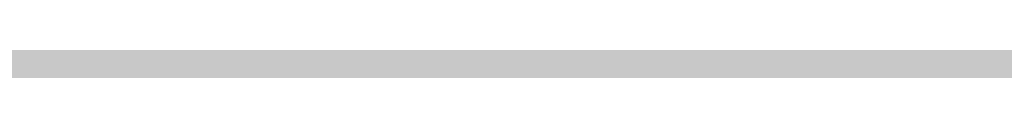
# Model space of a CAD drawing. Units: millimetres. Extents: x 0 to 2267, y 0 to 1823.
# Tile 125 of 256: x 1600.369 to 1605.705, y 1232.264 to 1232.332. Entities that reach past the tile are written whole.
import ezdxf

# ---------------------------------------------------------------- set-up
doc = ezdxf.new("R2010")
doc.units = ezdxf.units.MM
doc.header["$MEASUREMENT"] = 0
doc.layers.add('M-HATC', color=252, linetype='Continuous', lineweight=18)

msp = doc.modelspace()

# ---------------------------------------------------------------- hatches: boundary and pattern name
at = {"layer": 'M-HATC'}
h = msp.add_hatch(color=256, dxfattribs=at)
h.dxf.hatch_style = 1
h.paths.add_polyline_path([(2065.771, 1618.062, 0.236068), (2055.771, 1638.062), (1381.0868, 1638.062, 0.236068), (1371.0868, 1618.062), (1371.0868, 1603.062), (2055.771, 1603.062), (2065.771, 1603.062)])
h.paths.add_polyline_path([(2062.7718, 1550.2964), (2062.7718, 1560.2964), (1374.086, 1560.2964), (1374.086, 1550.2964), (1374.086, 1540.2964), (1384.086, 1540.2964), (1389.086, 1540.2964), (2062.7718, 1540.2964)])
h.paths.add_polyline_path([(1930.9289, 1282.7656), (1505.9289, 1282.7656), (1587.6276, 1235.5968, 0.131652), (1600.1276, 1232.2475), (1836.7302, 1232.2475, 0.131652), (1849.2302, 1235.5968)])
h.paths.add_polyline_path([(1930.9289, 1117.4171), (1905.9289, 1117.4171), (1505.9289, 1117.4171), (1505.9289, 1077.4171), (1930.9289, 1077.4171)])
h = msp.add_hatch(color=256, dxfattribs=at)
h.dxf.hatch_style = 1
h.paths.add_polyline_path([(2055.771, 1603.062), (1381.0868, 1603.062), (1381.0868, 1598.062), (2055.771, 1598.062)])
h.paths.add_polyline_path([(2055.771, 1598.062), (1381.0868, 1598.062), (1381.0868, 1593.062), (2055.771, 1593.062)])
h.paths.add_polyline_path([(2051.3074, 1536.7609), (1385.5504, 1536.7609), (1385.5504, 1526.7609), (1387.5504, 1526.7609), (1388.5366, 1525.0528), (1385.3319, 1521.2335), (1385.3319, 1521.2226), (2050.2542, 1522.7491), (2048.3212, 1525.0528), (2049.3074, 1526.7609), (2051.3074, 1526.7609)])
edge = h.paths.add_edge_path()
edge.add_arc((1847.5345, 1379.1492), 135, 222.603061, 222.890851, ccw=False)
edge.add_line((1748.1663, 1287.7656), (1683.0921, 1287.7656))
edge.add_arc((1583.7239, 1379.1492), 135, 317.109149, 317.396939, ccw=False)
edge.add_arc((1678.9686, 1290.6707), 5, 222.8909, 317.1091, ccw=False)
edge.add_arc((1774.2133, 1379.1492), 135, 222.603061, 222.890851, ccw=False)
edge.add_line((1674.8451, 1287.7656), (1609.7709, 1287.7656))
edge.add_arc((1510.4027, 1379.1492), 135, 317.109149, 317.396939, ccw=False)
edge.add_arc((1605.6474, 1290.6707), 5, 222.8909, 317.1091, ccw=False)
edge.add_arc((1700.8921, 1379.1492), 135, 222.603061, 222.890851, ccw=False)
edge.add_line((1601.5239, 1287.7656), (1536.4497, 1287.7656))
edge.add_arc((1437.0815, 1379.1492), 135, 317.109149, 317.396939, ccw=False)
edge.add_arc((1532.3262, 1290.6707), 5, 222.8909, 317.1091, ccw=False)
edge.add_arc((1627.5709, 1379.1492), 135, 222.603061, 222.890851, ccw=False)
edge.add_line((1528.2027, 1287.7656), (1505.9289, 1287.7656))
edge.add_spline(control_points=[(1505.9289, 1287.7656), (1504.2622, 1287.7656), (1504.2622, 1282.7656), (1505.9289, 1282.7656)], knot_values=[0, 0, 0, 0, 5, 5, 5, 5], degree=3, periodic=0)
edge.add_line((1505.9289, 1282.7656), (1930.9289, 1282.7656))
edge.add_spline(control_points=[(1930.9289, 1282.7656), (1932.5956, 1282.7656), (1932.5956, 1287.7656), (1930.9289, 1287.7656)], knot_values=[0, 0, 0, 0, 5, 5, 5, 5], degree=3, periodic=0)
edge.add_line((1930.9289, 1287.7656), (1903.0557, 1287.7656))
edge.add_arc((1803.6875, 1379.1492), 135, 317.109149, 317.396939, ccw=False)
edge.add_arc((1898.9322, 1290.6707), 5, 222.8909, 317.1091, ccw=False)
edge.add_arc((1994.1769, 1379.1492), 135, 222.603061, 222.890851, ccw=False)
edge.add_line((1894.8087, 1287.7656), (1829.7345, 1287.7656))
edge.add_arc((1730.3663, 1379.1492), 135, 317.109149, 317.396939, ccw=False)
edge.add_arc((1825.611, 1290.6707), 5, 222.8909, 317.1091, ccw=False)
edge.add_arc((1920.8557, 1379.1492), 135, 222.603061, 222.890851, ccw=False)
edge.add_line((1821.4875, 1287.7656), (1756.4133, 1287.7656))
edge.add_arc((1657.0451, 1379.1492), 135, 317.109149, 317.396939, ccw=False)
edge.add_arc((1752.2898, 1290.6707), 5, 222.8909, 317.1091, ccw=False)
edge = h.paths.add_edge_path()
edge.add_spline(control_points=[(1843.4289, 1227.2475), (1845.0956, 1227.2475), (1845.0956, 1232.2475), (1843.4289, 1232.2475)], knot_values=[0, 0, 0, 0, 5, 5, 5, 5], degree=3, periodic=0)
edge.add_line((1843.4289, 1232.2475), (1593.4289, 1232.2475))
edge.add_spline(control_points=[(1593.4289, 1232.2475), (1591.7622, 1232.2475), (1591.7622, 1227.2475), (1593.4289, 1227.2475)], knot_values=[0, 0, 0, 0, 5, 5, 5, 5], degree=3, periodic=0)
edge.add_line((1593.4289, 1227.2475), (1843.4289, 1227.2475))
h.paths.add_polyline_path([(1905.9289, 1127.4171), (1530.9289, 1127.4171, 0.414214), (1520.9289, 1117.4171), (1530.9289, 1117.4171), (1915.9289, 1117.4171, 0.414214)])
edge = h.paths.add_edge_path()
edge.add_arc((1397.0858, 1498.4078), 12.7299, 90.78215, 190.87871, ccw=False)
edge.add_line((1396.912, 1511.1365), (1428.0097, 1511.3488))
edge.add_line((1428.0097, 1511.3488), (1433.0097, 1511.3488))
edge.add_line((1433.0097, 1511.3488), (1434.439, 1511.3488))
edge.add_arc((1419.474, 1498.0804), 20, 41.561, 74.08211)
edge.add_line((1424.9592, 1517.3135), (1399.9351, 1517.2561))
edge.add_spline(control_points=[(1399.9307, 1517.2561), (1399.884, 1517.2131), (1399.8328, 1517.1689), (1399.7774, 1517.1236)], knot_values=[11.567499, 11.567499, 11.567499, 11.567499, 11.814249, 11.814249, 11.814249, 11.814249], degree=3, periodic=0)
edge.add_spline(control_points=[(1399.6328, 1517.0099), (1399.5831, 1516.9721), (1399.5307, 1516.9338), (1399.4759, 1516.8947)], knot_values=[11.167718, 11.167718, 11.167718, 11.167718, 11.365188, 11.365188, 11.365188, 11.365188], degree=3, periodic=0)
edge.add_spline(control_points=[(1399.3398, 1516.8001), (1399.1514, 1516.6719), (1398.9384, 1516.5377), (1398.704, 1516.3994)], knot_values=[10.376405, 10.376405, 10.376405, 10.376405, 11.00994, 11.00994, 11.00994, 11.00994], degree=3, periodic=0)
edge.add_spline(control_points=[(1398.6572, 1516.3719), (1398.5789, 1516.326), (1398.4983, 1516.2797), (1398.4155, 1516.2331)], knot_values=[10.125175, 10.125175, 10.125175, 10.125175, 10.334406, 10.334406, 10.334406, 10.334406], degree=3, periodic=0)
edge.add_spline(control_points=[(1398.2642, 1516.1487), (1398.196, 1516.1111), (1398.1263, 1516.0732), (1398.0555, 1516.0351)], knot_values=[9.832246, 9.832246, 9.832246, 9.832246, 9.999658, 9.999658, 9.999658, 9.999658], degree=3, periodic=0)
edge.add_spline(control_points=[(1397.9987, 1516.0048), (1397.7312, 1515.8621), (1397.446, 1515.7171), (1397.1466, 1515.5714)], knot_values=[9.161808, 9.161808, 9.161808, 9.161808, 9.787769, 9.787769, 9.787769, 9.787769], degree=3, periodic=0)
edge.add_spline(control_points=[(1397.1466, 1515.5714), (1396.8418, 1515.423), (1396.5222, 1515.274), (1396.1914, 1515.1262)], knot_values=[8.524455, 8.524455, 8.524455, 8.524455, 9.161808, 9.161808, 9.161808, 9.161808], degree=3, periodic=0)
edge.add_spline(control_points=[(1396.0777, 1515.0756), (1395.9854, 1515.0348), (1395.8922, 1514.994), (1395.7983, 1514.9534)], knot_values=[8.275193, 8.275193, 8.275193, 8.275193, 8.451726, 8.451726, 8.451726, 8.451726], degree=3, periodic=0)
edge.add_spline(control_points=[(1395.6018, 1514.8691), (1395.4997, 1514.8257), (1395.3968, 1514.7824), (1395.2932, 1514.7394)], knot_values=[7.962917, 7.962917, 7.962917, 7.962917, 8.152764, 8.152764, 8.152764, 8.152764], degree=3, periodic=0)
edge.add_spline(control_points=[(1395.2116, 1514.7057), (1394.8278, 1514.5475), (1394.4345, 1514.3929), (1394.0364, 1514.2442)], knot_values=[7.21254, 7.21254, 7.21254, 7.21254, 7.913148, 7.913148, 7.913148, 7.913148], degree=3, periodic=0)
edge.add_spline(control_points=[(1394.0364, 1514.2442), (1393.7076, 1514.1214), (1393.3754, 1514.0027), (1393.0427, 1513.8895)], knot_values=[6.633733, 6.633733, 6.633733, 6.633733, 7.21254, 7.21254, 7.21254, 7.21254], degree=3, periodic=0)
edge.add_spline(control_points=[(1392.8214, 1513.815), (1392.7198, 1513.7812), (1392.6181, 1513.7479), (1392.5166, 1513.7152)], knot_values=[6.328796, 6.328796, 6.328796, 6.328796, 6.505493, 6.505493, 6.505493, 6.505493], degree=3, periodic=0)
edge.add_spline(control_points=[(1392.5166, 1513.7152), (1392.3187, 1513.6515), (1392.1212, 1513.59), (1391.9244, 1513.531)], knot_values=[5.984605, 5.984605, 5.984605, 5.984605, 6.328796, 6.328796, 6.328796, 6.328796], degree=3, periodic=0)
edge.add_spline(control_points=[(1391.7915, 1513.4915), (1391.3122, 1513.3501), (1390.8384, 1513.2239), (1390.3784, 1513.1171)], knot_values=[5.066697, 5.066697, 5.066697, 5.066697, 5.907055, 5.907055, 5.907055, 5.907055], degree=3, periodic=0)
edge.add_spline(control_points=[(1390.3784, 1513.1171), (1390.1797, 1513.071), (1389.9836, 1513.0284), (1389.7907, 1512.9899)], knot_values=[4.70367, 4.70367, 4.70367, 4.70367, 5.066695, 5.066695, 5.066695, 5.066695], degree=3, periodic=0)
edge.add_spline(control_points=[(1389.422, 1512.9204), (1389.2459, 1512.8892), (1389.0729, 1512.8617), (1388.9036, 1512.8381)], knot_values=[4.130571, 4.130571, 4.130571, 4.130571, 4.469816, 4.469816, 4.469816, 4.469816], degree=3, periodic=0)
edge.add_spline(control_points=[(1388.9036, 1512.8381), (1388.591, 1512.7946), (1388.2911, 1512.7644), (1388.0071, 1512.7494)], knot_values=[3.504031, 3.504031, 3.504031, 3.504031, 4.130571, 4.130571, 4.130571, 4.130571], degree=3, periodic=0)
edge.add_spline(control_points=[(1387.9356, 1512.7459), (1387.8538, 1512.7423), (1387.7733, 1512.74), (1387.6944, 1512.739)], knot_values=[3.268866, 3.268866, 3.268866, 3.268866, 3.451164, 3.451164, 3.451164, 3.451164], degree=3, periodic=0)
edge.add_spline(control_points=[(1387.3351, 1512.7443), (1387.2076, 1512.7499), (1387.0847, 1512.7597), (1386.967, 1512.7739)], knot_values=[2.670686, 2.670686, 2.670686, 2.670686, 2.984, 2.984, 2.984, 2.984], degree=3, periodic=0)
edge.add_spline(control_points=[(1386.8327, 1512.7922), (1386.8209, 1512.7941), (1386.8092, 1512.7959), (1386.7975, 1512.7979)], knot_values=[2.516981, 2.516981, 2.516981, 2.516981, 2.549528, 2.549528, 2.549528, 2.549528], degree=3, periodic=0)
edge.add_spline(control_points=[(1386.4526, 1512.8735), (1386.4257, 1512.881), (1386.3993, 1512.889), (1386.3733, 1512.8972)], knot_values=[2.095869, 2.095869, 2.095869, 2.095869, 2.17941, 2.17941, 2.17941, 2.17941], degree=3, periodic=0)
edge.add_spline(control_points=[(1386.0691, 1513.0189), (1386.0634, 1513.0217), (1386.0577, 1513.0246), (1386.052, 1513.0275)], knot_values=[1.72453, 1.72453, 1.72453, 1.72453, 1.745933, 1.745933, 1.745933, 1.745933], degree=3, periodic=0)
edge.add_arc((1399.474, 1498.0804), 20, 131.82432, 180)
edge.add_arc((1630.3336, 1505.5484), 250.9708, 181.705176, 236.427975)
edge.add_arc((1605.3399, 1483.3044), 218.7822, 238.660829, 243.34961)
edge.add_arc((1647.0911, 1510.3592), 262.8986, 183.129836, 237.853442, ccw=False)
h.paths.add_polyline_path([(1406.5369, 1391.9644, 0.149382), (1491.5506, 1296.4418, -0.129517)], flags=17)
edge = h.paths.add_edge_path()
edge.add_arc((2037.3838, 1498.0804), 20, 0, 48.26587)
edge.add_spline(control_points=[(2050.6973, 1513.0052), (2050.6512, 1512.9847), (2050.6034, 1512.9655), (2050.5539, 1512.9477)], knot_values=[1.835652, 1.835652, 1.835652, 1.835652, 2.000781, 2.000781, 2.000781, 2.000781], degree=3, periodic=0)
edge.add_spline(control_points=[(2050.4616, 1512.9166), (2050.479, 1512.9221), (2050.4963, 1512.9277), (2050.5133, 1512.9335)], knot_values=[2.045477, 2.045477, 2.045477, 2.045477, 2.101389, 2.101389, 2.101389, 2.101389], degree=3, periodic=0)
edge.add_spline(control_points=[(2050.129, 1512.8342), (2050.1984, 1512.8473), (2050.2657, 1512.8623), (2050.3308, 1512.8792)], knot_values=[2.237629, 2.237629, 2.237629, 2.237629, 2.435841, 2.435841, 2.435841, 2.435841], degree=3, periodic=0)
edge.add_spline(control_points=[(2050.0946, 1512.8278), (2050.1061, 1512.8299), (2050.1176, 1512.832), (2050.129, 1512.8342)], knot_values=[2.435841, 2.435841, 2.435841, 2.435841, 2.468321, 2.468321, 2.468321, 2.468321], degree=3, periodic=0)
edge.add_spline(control_points=[(2049.7843, 1512.7851), (2049.8552, 1512.7922), (2049.9243, 1512.8008), (2049.9917, 1512.8109)], knot_values=[2.563852, 2.563852, 2.563852, 2.563852, 2.748541, 2.748541, 2.748541, 2.748541], degree=3, periodic=0)
edge.add_spline(control_points=[(2049.4052, 1512.7617), (2049.5364, 1512.7653), (2049.6629, 1512.773), (2049.7843, 1512.7851)], knot_values=[2.748541, 2.748541, 2.748541, 2.748541, 3.064882, 3.064882, 3.064882, 3.064882], degree=3, periodic=0)
edge.add_spline(control_points=[(2049.1698, 1512.7597), (2049.2336, 1512.7591), (2049.2965, 1512.7594), (2049.3584, 1512.7606)], knot_values=[3.102309, 3.102309, 3.102309, 3.102309, 3.2503, 3.2503, 3.2503, 3.2503], degree=3, periodic=0)
edge.add_spline(control_points=[(2048.8573, 1512.7691), (2048.9638, 1512.7638), (2049.068, 1512.7606), (2049.1698, 1512.7597)], knot_values=[3.2503, 3.2503, 3.2503, 3.2503, 3.486069, 3.486069, 3.486069, 3.486069], degree=3, periodic=0)
edge.add_spline(control_points=[(2048.6924, 1512.7789), (2048.3729, 1512.8009), (2048.0345, 1512.8411), (2047.6817, 1512.897)], knot_values=[3.606429, 3.606429, 3.606429, 3.606429, 4.2989, 4.2989, 4.2989, 4.2989], degree=3, periodic=0)
edge.add_spline(control_points=[(2047.6817, 1512.897), (2047.5458, 1512.9185), (2047.4077, 1512.9424), (2047.2678, 1512.9685)], knot_values=[4.2989, 4.2989, 4.2989, 4.2989, 4.565769, 4.565769, 4.565769, 4.565769], degree=3, periodic=0)
edge.add_spline(control_points=[(2047.2678, 1512.9685), (2047.1449, 1512.9914), (2047.0207, 1513.016), (2046.8951, 1513.0422)], knot_values=[4.565769, 4.565769, 4.565769, 4.565769, 4.799971, 4.799971, 4.799971, 4.799971], degree=3, periodic=0)
edge.add_spline(control_points=[(2046.8951, 1513.0422), (2046.5286, 1513.1188), (2046.1513, 1513.209), (2045.7676, 1513.3107)], knot_values=[4.799971, 4.799971, 4.799971, 4.799971, 5.483718, 5.483718, 5.483718, 5.483718], degree=3, periodic=0)
edge.add_spline(control_points=[(2045.7676, 1513.3107), (2045.3724, 1513.4154), (2044.9704, 1513.5322), (2044.5662, 1513.6588)], knot_values=[5.483718, 5.483718, 5.483718, 5.483718, 6.187866, 6.187866, 6.187866, 6.187866], degree=3, periodic=0)
edge.add_spline(control_points=[(2044.5662, 1513.6588), (2044.4149, 1513.7061), (2044.2633, 1513.7549), (2044.1116, 1513.8048)], knot_values=[6.187866, 6.187866, 6.187866, 6.187866, 6.451551, 6.451551, 6.451551, 6.451551], degree=3, periodic=0)
edge.add_spline(control_points=[(2044.1116, 1513.8048), (2043.9967, 1513.8427), (2043.8817, 1513.8813), (2043.7668, 1513.9205)], knot_values=[6.451551, 6.451551, 6.451551, 6.451551, 6.651434, 6.651434, 6.651434, 6.651434], degree=3, periodic=0)
edge.add_spline(control_points=[(2043.7668, 1513.9205), (2043.3716, 1514.0554), (2042.9774, 1514.1979), (2042.5886, 1514.3458)], knot_values=[6.651434, 6.651434, 6.651434, 6.651434, 7.338879, 7.338879, 7.338879, 7.338879], degree=3, periodic=0)
edge.add_spline(control_points=[(2042.5886, 1514.3458), (2042.1643, 1514.5071), (2041.7465, 1514.6749), (2041.3409, 1514.846)], knot_values=[7.338879, 7.338879, 7.338879, 7.338879, 8.089209, 8.089209, 8.089209, 8.089209], degree=3, periodic=0)
edge.add_spline(control_points=[(2041.3409, 1514.846), (2041.1028, 1514.9465), (2040.869, 1515.0481), (2040.6405, 1515.1502)], knot_values=[8.089209, 8.089209, 8.089209, 8.089209, 8.529587, 8.529587, 8.529587, 8.529587], degree=3, periodic=0)
edge.add_spline(control_points=[(2040.51, 1515.2089), (2040.0824, 1515.4022), (2039.6747, 1515.5971), (2039.295, 1515.7894)], knot_values=[8.613818, 8.613818, 8.613818, 8.613818, 9.44571, 9.44571, 9.44571, 9.44571], degree=3, periodic=0)
edge.add_spline(control_points=[(2039.295, 1515.7894), (2039.0618, 1515.9075), (2038.8391, 1516.0246), (2038.6288, 1516.1398)], knot_values=[9.44571, 9.44571, 9.44571, 9.44571, 9.956404, 9.956404, 9.956404, 9.956404], degree=3, periodic=0)
edge.add_spline(control_points=[(2038.6288, 1516.1398), (2038.5187, 1516.2001), (2038.4121, 1516.2598), (2038.309, 1516.3189)], knot_values=[9.956404, 9.956404, 9.956404, 9.956404, 10.223542, 10.223542, 10.223542, 10.223542], degree=3, periodic=0)
edge.add_spline(control_points=[(2038.309, 1516.3189), (2038.2138, 1516.3735), (2038.1216, 1516.4276), (2038.0328, 1516.481)], knot_values=[10.223542, 10.223542, 10.223542, 10.223542, 10.47051, 10.47051, 10.47051, 10.47051], degree=3, periodic=0)
edge.add_spline(control_points=[(2038.0328, 1516.481), (2037.7855, 1516.6296), (2037.5639, 1516.773), (2037.3722, 1516.909)], knot_values=[10.47051, 10.47051, 10.47051, 10.47051, 11.15767, 11.15767, 11.15767, 11.15767], degree=3, periodic=0)
edge.add_spline(control_points=[(2037.3722, 1516.909), (2037.2789, 1516.9752), (2037.1927, 1517.0396), (2037.1142, 1517.102)], knot_values=[11.15767, 11.15767, 11.15767, 11.15767, 11.49227, 11.49227, 11.49227, 11.49227], degree=3, periodic=0)
edge.add_spline(control_points=[(2036.8564, 1517.3259), (2036.9148, 1517.2692), (2036.9814, 1517.2103), (2037.0557, 1517.1492)], knot_values=[11.577341, 11.577341, 11.577341, 11.577341, 11.91035, 11.91035, 11.91035, 11.91035], degree=3, periodic=0)
edge.add_spline(control_points=[(2036.8074, 1517.3748), (2036.823, 1517.3587), (2036.8393, 1517.3424), (2036.8564, 1517.3259)], knot_values=[11.91035, 11.91035, 11.91035, 11.91035, 12.007402, 12.007402, 12.007402, 12.007402], degree=3, periodic=0)
edge.add_spline(control_points=[(2036.7017, 1517.494), (2036.7104, 1517.483), (2036.7196, 1517.4719), (2036.7291, 1517.4606)], knot_values=[12.184155, 12.184155, 12.184155, 12.184155, 12.255409, 12.255409, 12.255409, 12.255409], degree=3, periodic=0)
edge.add_spline(control_points=[(2036.6159, 1517.6205), (2036.62, 1517.613), (2036.6243, 1517.6055), (2036.6289, 1517.5979)], knot_values=[12.487913, 12.487913, 12.487913, 12.487913, 12.541035, 12.541035, 12.541035, 12.541035], degree=3, periodic=0)
edge.add_spline(control_points=[(2036.5635, 1517.786), (2036.5637, 1517.7794), (2036.5642, 1517.7726), (2036.565, 1517.7658)], knot_values=[12.911761, 12.911761, 12.911761, 12.911761, 12.968286, 12.968286, 12.968286, 12.968286], degree=3, periodic=0)
edge.add_spline(control_points=[(2036.6166, 1517.9304), (2036.6125, 1517.9259), (2036.6086, 1517.9212), (2036.6049, 1517.9165)], knot_values=[13.382527, 13.382527, 13.382527, 13.382527, 13.433791, 13.433791, 13.433791, 13.433791], degree=3, periodic=0)
edge.add_spline(control_points=[(2036.749, 1518.017), (2036.7361, 1518.0116), (2036.7239, 1518.006), (2036.7124, 1518.0002)], knot_values=[13.726299, 13.726299, 13.726299, 13.726299, 13.809928, 13.809928, 13.809928, 13.809928], degree=3, periodic=0)
edge.add_spline(control_points=[(2036.8604, 1518.0528), (2036.8386, 1518.0474), (2036.8181, 1518.0416), (2036.7988, 1518.0353)], knot_values=[13.910887, 13.910887, 13.910887, 13.910887, 14.02153, 14.02153, 14.02153, 14.02153], degree=3, periodic=0)
edge.add_line((2036.9639, 1518.0804), (2032.3838, 1518.0804))
edge.add_line((2032.3838, 1518.0804), (2027.3838, 1518.0804))
edge.add_line((2027.3838, 1518.0804), (2022.3838, 1518.0804))
edge.add_line((2022.3838, 1518.0804), (2017.3838, 1518.0804))
edge.add_arc((2017.3838, 1498.0804), 20, 90, 138.439)
edge.add_line((2002.4188, 1511.3488), (2003.8481, 1511.3488))
edge.add_line((2003.8481, 1511.3488), (2008.8481, 1511.3488))
edge.add_line((2008.8481, 1511.3488), (2039.772, 1511.1377))
edge.add_arc((2039.772, 1498.4078), 12.7299, -10.87871, 90, ccw=False)
edge.add_arc((1789.7668, 1510.3592), 262.8986, 302.146558, 356.870164, ccw=False)
edge.add_arc((1831.5179, 1483.3044), 218.7822, 296.65039, 301.339171)
edge.add_arc((1806.5242, 1505.5484), 250.9708, 303.572025, 358.294824)
h.paths.add_polyline_path([(2030.321, 1391.9644, -0.129517), (1945.3072, 1296.4418, 0.149382)], flags=17)
edge = h.paths.add_edge_path()
edge.add_spline(control_points=[(2037.2464, 1518.0821), (2037.2898, 1518.081), (2037.3355, 1518.0804), (2037.3838, 1518.0804)], knot_values=[0.000012, 0.000012, 0.000012, 0.000012, 0.144754, 0.144754, 0.144754, 0.144754], degree=3, periodic=0)
edge.add_line((2037.3357, 1518.0804), (2037.0096, 1518.0804))
edge.add_spline(control_points=[(2037.0096, 1518.0804), (2036.9822, 1518.0768), (2036.956, 1518.0727), (2036.9312, 1518.0681)], knot_values=[14.13465, 14.13465, 14.13465, 14.13465, 14.247197, 14.247197, 14.247197, 14.247197], degree=3, periodic=0)
edge.add_spline(control_points=[(2036.9312, 1518.0681), (2036.9276, 1518.0674), (2036.9241, 1518.0667), (2036.9205, 1518.0661)], knot_values=[14.118315, 14.118315, 14.118315, 14.118315, 14.13465, 14.13465, 14.13465, 14.13465], degree=3, periodic=0)
edge.add_spline(control_points=[(2036.9205, 1518.0661), (2036.9118, 1518.0644), (2036.9032, 1518.0626), (2036.8948, 1518.0608)], knot_values=[14.078086, 14.078086, 14.078086, 14.078086, 14.118315, 14.118315, 14.118315, 14.118315], degree=3, periodic=0)
edge.add_spline(control_points=[(2036.8948, 1518.0608), (2036.883, 1518.0583), (2036.8716, 1518.0556), (2036.8604, 1518.0528)], knot_values=[14.02153, 14.02153, 14.02153, 14.02153, 14.078086, 14.078086, 14.078086, 14.078086], degree=3, periodic=0)
edge.add_spline(control_points=[(2036.8604, 1518.0528), (2036.8386, 1518.0474), (2036.8181, 1518.0416), (2036.7988, 1518.0353)], knot_values=[13.910887, 13.910887, 13.910887, 13.910887, 14.02153, 14.02153, 14.02153, 14.02153], degree=3, periodic=0)
edge.add_spline(control_points=[(2036.7988, 1518.0353), (2036.7981, 1518.035), (2036.7974, 1518.0348), (2036.7967, 1518.0346)], knot_values=[13.906906, 13.906906, 13.906906, 13.906906, 13.910887, 13.910887, 13.910887, 13.910887], degree=3, periodic=0)
edge.add_spline(control_points=[(2036.7967, 1518.0346), (2036.7882, 1518.0318), (2036.7799, 1518.0289), (2036.7719, 1518.0259)], knot_values=[13.857826, 13.857826, 13.857826, 13.857826, 13.906906, 13.906906, 13.906906, 13.906906], degree=3, periodic=0)
edge.add_spline(control_points=[(2036.7719, 1518.0259), (2036.764, 1518.023), (2036.7564, 1518.02), (2036.749, 1518.017)], knot_values=[13.809928, 13.809928, 13.809928, 13.809928, 13.857826, 13.857826, 13.857826, 13.857826], degree=3, periodic=0)
edge.add_spline(control_points=[(2036.749, 1518.017), (2036.7361, 1518.0116), (2036.7239, 1518.006), (2036.7124, 1518.0002)], knot_values=[13.726299, 13.726299, 13.726299, 13.726299, 13.809928, 13.809928, 13.809928, 13.809928], degree=3, periodic=0)
edge.add_spline(control_points=[(2036.7124, 1518.0002), (2036.7121, 1518), (2036.7118, 1517.9999), (2036.7115, 1517.9997)], knot_values=[13.723993, 13.723993, 13.723993, 13.723993, 13.726299, 13.726299, 13.726299, 13.726299], degree=3, periodic=0)
edge.add_spline(control_points=[(2036.7115, 1517.9997), (2036.7063, 1517.9971), (2036.7013, 1517.9944), (2036.6965, 1517.9917)], knot_values=[13.686536, 13.686536, 13.686536, 13.686536, 13.723993, 13.723993, 13.723993, 13.723993], degree=3, periodic=0)
edge.add_spline(control_points=[(2036.6965, 1517.9917), (2036.6919, 1517.9891), (2036.6874, 1517.9865), (2036.6831, 1517.9839)], knot_values=[13.651251, 13.651251, 13.651251, 13.651251, 13.686536, 13.686536, 13.686536, 13.686536], degree=3, periodic=0)
edge.add_spline(control_points=[(2036.6831, 1517.9839), (2036.6764, 1517.9798), (2036.67, 1517.9757), (2036.6639, 1517.9714)], knot_values=[13.596804, 13.596804, 13.596804, 13.596804, 13.651251, 13.651251, 13.651251, 13.651251], degree=3, periodic=0)
edge.add_spline(control_points=[(2036.6639, 1517.9714), (2036.6636, 1517.9712), (2036.6633, 1517.9709), (2036.6629, 1517.9707)], knot_values=[13.593956, 13.593956, 13.593956, 13.593956, 13.596804, 13.596804, 13.596804, 13.596804], degree=3, periodic=0)
edge.add_spline(control_points=[(2036.6629, 1517.9707), (2036.6603, 1517.9689), (2036.6577, 1517.967), (2036.6552, 1517.9651)], knot_values=[13.570322, 13.570322, 13.570322, 13.570322, 13.593956, 13.593956, 13.593956, 13.593956], degree=3, periodic=0)
edge.add_spline(control_points=[(2036.6552, 1517.9651), (2036.6525, 1517.9631), (2036.6499, 1517.9611), (2036.6474, 1517.9591)], knot_values=[13.545477, 13.545477, 13.545477, 13.545477, 13.570322, 13.570322, 13.570322, 13.570322], degree=3, periodic=0)
edge.add_spline(control_points=[(2036.6474, 1517.9591), (2036.6472, 1517.9589), (2036.6471, 1517.9588), (2036.6469, 1517.9587)], knot_values=[13.543931, 13.543931, 13.543931, 13.543931, 13.545477, 13.545477, 13.545477, 13.545477], degree=3, periodic=0)
edge.add_spline(control_points=[(2036.6469, 1517.9587), (2036.6412, 1517.9541), (2036.6358, 1517.9494), (2036.6307, 1517.9447)], knot_values=[13.488237, 13.488237, 13.488237, 13.488237, 13.543931, 13.543931, 13.543931, 13.543931], degree=3, periodic=0)
edge.add_spline(control_points=[(2036.6307, 1517.9447), (2036.6282, 1517.9423), (2036.6257, 1517.9399), (2036.6233, 1517.9374)], knot_values=[13.460307, 13.460307, 13.460307, 13.460307, 13.488237, 13.488237, 13.488237, 13.488237], degree=3, periodic=0)
edge.add_spline(control_points=[(2036.6233, 1517.9374), (2036.6215, 1517.9356), (2036.6198, 1517.9338), (2036.6181, 1517.932)], knot_values=[13.439712, 13.439712, 13.439712, 13.439712, 13.460307, 13.460307, 13.460307, 13.460307], degree=3, periodic=0)
edge.add_spline(control_points=[(2036.6181, 1517.932), (2036.6176, 1517.9315), (2036.6171, 1517.9309), (2036.6166, 1517.9304)], knot_values=[13.433791, 13.433791, 13.433791, 13.433791, 13.439712, 13.439712, 13.439712, 13.439712], degree=3, periodic=0)
edge.add_spline(control_points=[(2036.6166, 1517.9304), (2036.6125, 1517.9259), (2036.6086, 1517.9212), (2036.6049, 1517.9165)], knot_values=[13.382527, 13.382527, 13.382527, 13.382527, 13.433791, 13.433791, 13.433791, 13.433791], degree=3, periodic=0)
edge.add_spline(control_points=[(2036.6049, 1517.9165), (2036.6026, 1517.9135), (2036.6004, 1517.9104), (2036.5982, 1517.9074)], knot_values=[13.350017, 13.350017, 13.350017, 13.350017, 13.382527, 13.382527, 13.382527, 13.382527], degree=3, periodic=0)
edge.add_spline(control_points=[(2036.5982, 1517.9074), (2036.5972, 1517.9059), (2036.5962, 1517.9043), (2036.5952, 1517.9028)], knot_values=[13.333922, 13.333922, 13.333922, 13.333922, 13.350017, 13.350017, 13.350017, 13.350017], degree=3, periodic=0)
edge.add_spline(control_points=[(2036.5952, 1517.9028), (2036.5945, 1517.9018), (2036.5939, 1517.9009), (2036.5933, 1517.8999)], knot_values=[13.323828, 13.323828, 13.323828, 13.323828, 13.333922, 13.333922, 13.333922, 13.333922], degree=3, periodic=0)
edge.add_spline(control_points=[(2036.5933, 1517.8999), (2036.5905, 1517.8955), (2036.5879, 1517.8909), (2036.5855, 1517.8864)], knot_values=[13.277545, 13.277545, 13.277545, 13.277545, 13.323828, 13.323828, 13.323828, 13.323828], degree=3, periodic=0)
edge.add_spline(control_points=[(2036.5855, 1517.8864), (2036.5836, 1517.8827), (2036.5817, 1517.8789), (2036.5801, 1517.8751)], knot_values=[13.240119, 13.240119, 13.240119, 13.240119, 13.277545, 13.277545, 13.277545, 13.277545], degree=3, periodic=0)
edge.add_spline(control_points=[(2036.5801, 1517.8751), (2036.5795, 1517.8739), (2036.579, 1517.8727), (2036.5785, 1517.8715)], knot_values=[13.228211, 13.228211, 13.228211, 13.228211, 13.240119, 13.240119, 13.240119, 13.240119], degree=3, periodic=0)
edge.add_spline(control_points=[(2036.5785, 1517.8715), (2036.578, 1517.8702), (2036.5774, 1517.869), (2036.5769, 1517.8677)], knot_values=[13.215717, 13.215717, 13.215717, 13.215717, 13.228211, 13.228211, 13.228211, 13.228211], degree=3, periodic=0)
edge.add_spline(control_points=[(2036.5769, 1517.8677), (2036.5755, 1517.864), (2036.5741, 1517.8603), (2036.5729, 1517.8565)], knot_values=[13.179847, 13.179847, 13.179847, 13.179847, 13.215717, 13.215717, 13.215717, 13.215717], degree=3, periodic=0)
edge.add_spline(control_points=[(2036.5729, 1517.8565), (2036.5713, 1517.8515), (2036.5699, 1517.8464), (2036.5687, 1517.8413)], knot_values=[13.132017, 13.132017, 13.132017, 13.132017, 13.179847, 13.179847, 13.179847, 13.179847], degree=3, periodic=0)
edge.add_spline(control_points=[(2036.5687, 1517.8413), (2036.5684, 1517.8402), (2036.5682, 1517.8392), (2036.568, 1517.8382)], knot_values=[13.122482, 13.122482, 13.122482, 13.122482, 13.132017, 13.132017, 13.132017, 13.132017], degree=3, periodic=0)
edge.add_spline(control_points=[(2036.568, 1517.8382), (2036.5676, 1517.8363), (2036.5672, 1517.8345), (2036.5669, 1517.8327)], knot_values=[13.105592, 13.105592, 13.105592, 13.105592, 13.122482, 13.122482, 13.122482, 13.122482], degree=3, periodic=0)
edge.add_spline(control_points=[(2036.5669, 1517.8327), (2036.5662, 1517.8292), (2036.5657, 1517.8257), (2036.5652, 1517.8222)], knot_values=[13.074063, 13.074063, 13.074063, 13.074063, 13.105592, 13.105592, 13.105592, 13.105592], degree=3, periodic=0)
edge.add_spline(control_points=[(2036.5652, 1517.8222), (2036.5652, 1517.8222), (2036.5652, 1517.8222), (2036.5652, 1517.8222)], knot_values=[13.074043, 13.074043, 13.074043, 13.074043, 13.074063, 13.074063, 13.074063, 13.074063], degree=3, periodic=0)
edge.add_spline(control_points=[(2036.5652, 1517.8222), (2036.5644, 1517.8164), (2036.5639, 1517.8106), (2036.5636, 1517.8046)], knot_values=[13.021884, 13.021884, 13.021884, 13.021884, 13.074043, 13.074043, 13.074043, 13.074043], degree=3, periodic=0)
edge.add_spline(control_points=[(2036.5636, 1517.8046), (2036.5636, 1517.804), (2036.5636, 1517.8034), (2036.5635, 1517.8028)], knot_values=[13.01674, 13.01674, 13.01674, 13.01674, 13.021884, 13.021884, 13.021884, 13.021884], degree=3, periodic=0)
edge.add_spline(control_points=[(2036.5635, 1517.8028), (2036.5634, 1517.8005), (2036.5634, 1517.7982), (2036.5634, 1517.7958)], knot_values=[12.996438, 12.996438, 12.996438, 12.996438, 13.01674, 13.01674, 13.01674, 13.01674], degree=3, periodic=0)
edge.add_spline(control_points=[(2036.5634, 1517.7958), (2036.5633, 1517.7926), (2036.5634, 1517.7893), (2036.5635, 1517.786)], knot_values=[12.968286, 12.968286, 12.968286, 12.968286, 12.996438, 12.996438, 12.996438, 12.996438], degree=3, periodic=0)
edge.add_spline(control_points=[(2036.5635, 1517.786), (2036.5637, 1517.7794), (2036.5642, 1517.7726), (2036.565, 1517.7658)], knot_values=[12.911761, 12.911761, 12.911761, 12.911761, 12.968286, 12.968286, 12.968286, 12.968286], degree=3, periodic=0)
edge.add_spline(control_points=[(2036.565, 1517.7658), (2036.565, 1517.7657), (2036.565, 1517.7656), (2036.565, 1517.7656)], knot_values=[12.911017, 12.911017, 12.911017, 12.911017, 12.911761, 12.911761, 12.911761, 12.911761], degree=3, periodic=0)
edge.add_spline(control_points=[(2036.565, 1517.7656), (2036.5654, 1517.7625), (2036.5658, 1517.7593), (2036.5663, 1517.7562)], knot_values=[12.88528, 12.88528, 12.88528, 12.88528, 12.911017, 12.911017, 12.911017, 12.911017], degree=3, periodic=0)
edge.add_spline(control_points=[(2036.5663, 1517.7562), (2036.5667, 1517.7534), (2036.5672, 1517.7506), (2036.5677, 1517.7478)], knot_values=[12.862519, 12.862519, 12.862519, 12.862519, 12.88528, 12.88528, 12.88528, 12.88528], degree=3, periodic=0)
edge.add_spline(control_points=[(2036.5677, 1517.7478), (2036.5678, 1517.7474), (2036.5679, 1517.7469), (2036.568, 1517.7465)], knot_values=[12.858885, 12.858885, 12.858885, 12.858885, 12.862519, 12.862519, 12.862519, 12.862519], degree=3, periodic=0)
edge.add_spline(control_points=[(2036.568, 1517.7465), (2036.5692, 1517.7399), (2036.5707, 1517.7332), (2036.5724, 1517.7264)], knot_values=[12.8053, 12.8053, 12.8053, 12.8053, 12.858885, 12.858885, 12.858885, 12.858885], degree=3, periodic=0)
edge.add_spline(control_points=[(2036.5724, 1517.7264), (2036.5734, 1517.7226), (2036.5745, 1517.7187), (2036.5756, 1517.7149)], knot_values=[12.775176, 12.775176, 12.775176, 12.775176, 12.8053, 12.8053, 12.8053, 12.8053], degree=3, periodic=0)
edge.add_spline(control_points=[(2036.5756, 1517.7149), (2036.5763, 1517.7125), (2036.577, 1517.7102), (2036.5778, 1517.7078)], knot_values=[12.756759, 12.756759, 12.756759, 12.756759, 12.775176, 12.775176, 12.775176, 12.775176], degree=3, periodic=0)
edge.add_spline(control_points=[(2036.5778, 1517.7078), (2036.5781, 1517.7067), (2036.5784, 1517.7057), (2036.5787, 1517.7047)], knot_values=[12.748742, 12.748742, 12.748742, 12.748742, 12.756759, 12.756759, 12.756759, 12.756759], degree=3, periodic=0)
edge.add_spline(control_points=[(2036.5787, 1517.7047), (2036.5808, 1517.6983), (2036.5831, 1517.6919), (2036.5856, 1517.6854)], knot_values=[12.69959, 12.69959, 12.69959, 12.69959, 12.748742, 12.748742, 12.748742, 12.748742], degree=3, periodic=0)
edge.add_spline(control_points=[(2036.5856, 1517.6854), (2036.5876, 1517.68), (2036.5898, 1517.6746), (2036.5921, 1517.6692)], knot_values=[12.659038, 12.659038, 12.659038, 12.659038, 12.69959, 12.69959, 12.69959, 12.69959], degree=3, periodic=0)
edge.add_spline(control_points=[(2036.5921, 1517.6692), (2036.594, 1517.6648), (2036.5959, 1517.6605), (2036.5979, 1517.6561)], knot_values=[12.626806, 12.626806, 12.626806, 12.626806, 12.659038, 12.659038, 12.659038, 12.659038], degree=3, periodic=0)
edge.add_spline(control_points=[(2036.5979, 1517.6561), (2036.5984, 1517.6551), (2036.5989, 1517.6541), (2036.5993, 1517.6531)], knot_values=[12.619394, 12.619394, 12.619394, 12.619394, 12.626806, 12.626806, 12.626806, 12.626806], degree=3, periodic=0)
edge.add_spline(control_points=[(2036.5993, 1517.6531), (2036.6043, 1517.6424), (2036.6099, 1517.6315), (2036.6159, 1517.6205)], knot_values=[12.541039, 12.541039, 12.541039, 12.541039, 12.619394, 12.619394, 12.619394, 12.619394], degree=3, periodic=0)
edge.add_spline(control_points=[(2036.6159, 1517.6205), (2036.6159, 1517.6205), (2036.6159, 1517.6205), (2036.6159, 1517.6205)], knot_values=[12.541035, 12.541035, 12.541035, 12.541035, 12.541039, 12.541039, 12.541039, 12.541039], degree=3, periodic=0)
edge.add_spline(control_points=[(2036.6159, 1517.6205), (2036.62, 1517.613), (2036.6243, 1517.6055), (2036.6289, 1517.5979)], knot_values=[12.487913, 12.487913, 12.487913, 12.487913, 12.541035, 12.541035, 12.541035, 12.541035], degree=3, periodic=0)
edge.add_spline(control_points=[(2036.6289, 1517.5979), (2036.6326, 1517.5916), (2036.6365, 1517.5853), (2036.6406, 1517.5789)], knot_values=[12.443982, 12.443982, 12.443982, 12.443982, 12.487913, 12.487913, 12.487913, 12.487913], degree=3, periodic=0)
edge.add_spline(control_points=[(2036.6406, 1517.5789), (2036.6414, 1517.5776), (2036.6423, 1517.5763), (2036.6431, 1517.5749)], knot_values=[12.434996, 12.434996, 12.434996, 12.434996, 12.443982, 12.443982, 12.443982, 12.443982], degree=3, periodic=0)
edge.add_spline(control_points=[(2036.6431, 1517.5749), (2036.6531, 1517.5596), (2036.6639, 1517.5439), (2036.6756, 1517.528)], knot_values=[12.329647, 12.329647, 12.329647, 12.329647, 12.434996, 12.434996, 12.434996, 12.434996], degree=3, periodic=0)
edge.add_spline(control_points=[(2036.6756, 1517.528), (2036.6839, 1517.5168), (2036.6925, 1517.5055), (2036.7017, 1517.494)], knot_values=[12.255409, 12.255409, 12.255409, 12.255409, 12.329647, 12.329647, 12.329647, 12.329647], degree=3, periodic=0)
edge.add_spline(control_points=[(2036.7017, 1517.494), (2036.7104, 1517.483), (2036.7196, 1517.4719), (2036.7291, 1517.4606)], knot_values=[12.184155, 12.184155, 12.184155, 12.184155, 12.255409, 12.255409, 12.255409, 12.255409], degree=3, periodic=0)
edge.add_spline(control_points=[(2036.7291, 1517.4606), (2036.7436, 1517.4435), (2036.759, 1517.4262), (2036.7753, 1517.4085)], knot_values=[12.075961, 12.075961, 12.075961, 12.075961, 12.184155, 12.184155, 12.184155, 12.184155], degree=3, periodic=0)
edge.add_spline(control_points=[(2036.7753, 1517.4085), (2036.7763, 1517.4075), (2036.7773, 1517.4064), (2036.7783, 1517.4054)], knot_values=[12.069502, 12.069502, 12.069502, 12.069502, 12.075961, 12.075961, 12.075961, 12.075961], degree=3, periodic=0)
edge.add_spline(control_points=[(2036.7783, 1517.4054), (2036.7877, 1517.3953), (2036.7974, 1517.385), (2036.8074, 1517.3748)], knot_values=[12.007402, 12.007402, 12.007402, 12.007402, 12.069502, 12.069502, 12.069502, 12.069502], degree=3, periodic=0)
edge.add_spline(control_points=[(2036.8074, 1517.3748), (2036.823, 1517.3587), (2036.8393, 1517.3424), (2036.8564, 1517.3259)], knot_values=[11.91035, 11.91035, 11.91035, 11.91035, 12.007402, 12.007402, 12.007402, 12.007402], degree=3, periodic=0)
edge.add_spline(control_points=[(2036.8564, 1517.3259), (2036.9148, 1517.2692), (2036.9814, 1517.2103), (2037.0557, 1517.1492)], knot_values=[11.577341, 11.577341, 11.577341, 11.577341, 11.91035, 11.91035, 11.91035, 11.91035], degree=3, periodic=0)
edge.add_spline(control_points=[(2037.0557, 1517.1492), (2037.0747, 1517.1336), (2037.0942, 1517.1179), (2037.1142, 1517.102)], knot_values=[11.49227, 11.49227, 11.49227, 11.49227, 11.577341, 11.577341, 11.577341, 11.577341], degree=3, periodic=0)
edge.add_spline(control_points=[(2037.1142, 1517.102), (2037.1927, 1517.0396), (2037.2789, 1516.9752), (2037.3722, 1516.909)], knot_values=[11.15767, 11.15767, 11.15767, 11.15767, 11.49227, 11.49227, 11.49227, 11.49227], degree=3, periodic=0)
edge.add_spline(control_points=[(2037.3722, 1516.909), (2037.5639, 1516.773), (2037.7855, 1516.6296), (2038.0328, 1516.481)], knot_values=[10.47051, 10.47051, 10.47051, 10.47051, 11.15767, 11.15767, 11.15767, 11.15767], degree=3, periodic=0)
edge.add_spline(control_points=[(2038.0328, 1516.481), (2038.1216, 1516.4276), (2038.2138, 1516.3735), (2038.309, 1516.3189)], knot_values=[10.223542, 10.223542, 10.223542, 10.223542, 10.47051, 10.47051, 10.47051, 10.47051], degree=3, periodic=0)
edge.add_spline(control_points=[(2038.309, 1516.3189), (2038.4121, 1516.2598), (2038.5187, 1516.2001), (2038.6288, 1516.1398)], knot_values=[9.956404, 9.956404, 9.956404, 9.956404, 10.223542, 10.223542, 10.223542, 10.223542], degree=3, periodic=0)
edge.add_spline(control_points=[(2038.6288, 1516.1398), (2038.8391, 1516.0246), (2039.0618, 1515.9075), (2039.295, 1515.7894)], knot_values=[9.44571, 9.44571, 9.44571, 9.44571, 9.956404, 9.956404, 9.956404, 9.956404], degree=3, periodic=0)
edge.add_spline(control_points=[(2039.295, 1515.7894), (2039.6747, 1515.5971), (2040.0824, 1515.4022), (2040.51, 1515.2089)], knot_values=[8.613818, 8.613818, 8.613818, 8.613818, 9.44571, 9.44571, 9.44571, 9.44571], degree=3, periodic=0)
edge.add_spline(control_points=[(2040.51, 1515.2089), (2040.5533, 1515.1893), (2040.5968, 1515.1697), (2040.6405, 1515.1502)], knot_values=[8.529587, 8.529587, 8.529587, 8.529587, 8.613818, 8.613818, 8.613818, 8.613818], degree=3, periodic=0)
edge.add_spline(control_points=[(2040.6405, 1515.1502), (2040.869, 1515.0481), (2041.1028, 1514.9465), (2041.3409, 1514.846)], knot_values=[8.089209, 8.089209, 8.089209, 8.089209, 8.529587, 8.529587, 8.529587, 8.529587], degree=3, periodic=0)
edge.add_spline(control_points=[(2041.3409, 1514.846), (2041.7465, 1514.6749), (2042.1643, 1514.5071), (2042.5886, 1514.3458)], knot_values=[7.338879, 7.338879, 7.338879, 7.338879, 8.089209, 8.089209, 8.089209, 8.089209], degree=3, periodic=0)
edge.add_spline(control_points=[(2042.5886, 1514.3458), (2042.9774, 1514.1979), (2043.3716, 1514.0554), (2043.7668, 1513.9205)], knot_values=[6.651434, 6.651434, 6.651434, 6.651434, 7.338879, 7.338879, 7.338879, 7.338879], degree=3, periodic=0)
edge.add_spline(control_points=[(2043.7668, 1513.9205), (2043.8817, 1513.8813), (2043.9967, 1513.8427), (2044.1116, 1513.8048)], knot_values=[6.451551, 6.451551, 6.451551, 6.451551, 6.651434, 6.651434, 6.651434, 6.651434], degree=3, periodic=0)
edge.add_spline(control_points=[(2044.1116, 1513.8048), (2044.2633, 1513.7549), (2044.4149, 1513.7061), (2044.5662, 1513.6588)], knot_values=[6.187866, 6.187866, 6.187866, 6.187866, 6.451551, 6.451551, 6.451551, 6.451551], degree=3, periodic=0)
edge.add_spline(control_points=[(2044.5662, 1513.6588), (2044.9704, 1513.5322), (2045.3724, 1513.4154), (2045.7676, 1513.3107)], knot_values=[5.483718, 5.483718, 5.483718, 5.483718, 6.187866, 6.187866, 6.187866, 6.187866], degree=3, periodic=0)
edge.add_spline(control_points=[(2045.7676, 1513.3107), (2046.1513, 1513.209), (2046.5286, 1513.1188), (2046.8951, 1513.0422)], knot_values=[4.799971, 4.799971, 4.799971, 4.799971, 5.483718, 5.483718, 5.483718, 5.483718], degree=3, periodic=0)
edge.add_spline(control_points=[(2046.8951, 1513.0422), (2047.0207, 1513.016), (2047.1449, 1512.9914), (2047.2678, 1512.9685)], knot_values=[4.565769, 4.565769, 4.565769, 4.565769, 4.799971, 4.799971, 4.799971, 4.799971], degree=3, periodic=0)
edge.add_spline(control_points=[(2047.2678, 1512.9685), (2047.4077, 1512.9424), (2047.5458, 1512.9185), (2047.6817, 1512.897)], knot_values=[4.2989, 4.2989, 4.2989, 4.2989, 4.565769, 4.565769, 4.565769, 4.565769], degree=3, periodic=0)
edge.add_spline(control_points=[(2047.6817, 1512.897), (2048.0345, 1512.8411), (2048.3729, 1512.8009), (2048.6924, 1512.7789)], knot_values=[3.606429, 3.606429, 3.606429, 3.606429, 4.2989, 4.2989, 4.2989, 4.2989], degree=3, periodic=0)
edge.add_spline(control_points=[(2048.6924, 1512.7789), (2048.7479, 1512.7751), (2048.8029, 1512.7718), (2048.8573, 1512.7691)], knot_values=[3.486069, 3.486069, 3.486069, 3.486069, 3.606429, 3.606429, 3.606429, 3.606429], degree=3, periodic=0)
edge.add_spline(control_points=[(2048.8573, 1512.7691), (2048.9638, 1512.7638), (2049.068, 1512.7606), (2049.1698, 1512.7597)], knot_values=[3.2503, 3.2503, 3.2503, 3.2503, 3.486069, 3.486069, 3.486069, 3.486069], degree=3, periodic=0)
edge.add_spline(control_points=[(2049.1698, 1512.7597), (2049.2336, 1512.7591), (2049.2965, 1512.7594), (2049.3584, 1512.7606)], knot_values=[3.102309, 3.102309, 3.102309, 3.102309, 3.2503, 3.2503, 3.2503, 3.2503], degree=3, periodic=0)
edge.add_spline(control_points=[(2049.3584, 1512.7606), (2049.3741, 1512.7609), (2049.3897, 1512.7613), (2049.4052, 1512.7617)], knot_values=[3.064882, 3.064882, 3.064882, 3.064882, 3.102309, 3.102309, 3.102309, 3.102309], degree=3, periodic=0)
edge.add_spline(control_points=[(2049.4052, 1512.7617), (2049.5364, 1512.7653), (2049.6629, 1512.773), (2049.7843, 1512.7851)], knot_values=[2.748541, 2.748541, 2.748541, 2.748541, 3.064882, 3.064882, 3.064882, 3.064882], degree=3, periodic=0)
edge.add_spline(control_points=[(2049.7843, 1512.7851), (2049.8552, 1512.7922), (2049.9243, 1512.8008), (2049.9917, 1512.8109)], knot_values=[2.563852, 2.563852, 2.563852, 2.563852, 2.748541, 2.748541, 2.748541, 2.748541], degree=3, periodic=0)
edge.add_spline(control_points=[(2049.9917, 1512.8109), (2050.0265, 1512.8161), (2050.0608, 1512.8218), (2050.0946, 1512.8278)], knot_values=[2.468321, 2.468321, 2.468321, 2.468321, 2.563852, 2.563852, 2.563852, 2.563852], degree=3, periodic=0)
edge.add_spline(control_points=[(2050.0946, 1512.8278), (2050.1061, 1512.8299), (2050.1176, 1512.832), (2050.129, 1512.8342)], knot_values=[2.435841, 2.435841, 2.435841, 2.435841, 2.468321, 2.468321, 2.468321, 2.468321], degree=3, periodic=0)
edge.add_spline(control_points=[(2050.129, 1512.8342), (2050.1984, 1512.8473), (2050.2657, 1512.8623), (2050.3308, 1512.8792)], knot_values=[2.237629, 2.237629, 2.237629, 2.237629, 2.435841, 2.435841, 2.435841, 2.435841], degree=3, periodic=0)
edge.add_spline(control_points=[(2050.3308, 1512.8792), (2050.3754, 1512.8908), (2050.4191, 1512.9032), (2050.4616, 1512.9166)], knot_values=[2.101389, 2.101389, 2.101389, 2.101389, 2.237629, 2.237629, 2.237629, 2.237629], degree=3, periodic=0)
edge.add_spline(control_points=[(2050.4616, 1512.9166), (2050.479, 1512.9221), (2050.4963, 1512.9277), (2050.5133, 1512.9335)], knot_values=[2.045477, 2.045477, 2.045477, 2.045477, 2.101389, 2.101389, 2.101389, 2.101389], degree=3, periodic=0)
edge.add_spline(control_points=[(2050.5133, 1512.9335), (2050.527, 1512.9382), (2050.5405, 1512.9429), (2050.5539, 1512.9477)], knot_values=[2.000781, 2.000781, 2.000781, 2.000781, 2.045477, 2.045477, 2.045477, 2.045477], degree=3, periodic=0)
edge.add_spline(control_points=[(2050.5539, 1512.9477), (2050.6034, 1512.9655), (2050.6512, 1512.9847), (2050.6973, 1513.0052)], knot_values=[1.835652, 1.835652, 1.835652, 1.835652, 2.000781, 2.000781, 2.000781, 2.000781], degree=3, periodic=0)
edge.add_arc((2037.3838, 1498.0804), 20, 48.26587, 90.12993)
edge = h.paths.add_edge_path(flags=16)
edge.add_spline(control_points=[(1386.1389, 1512.9859), (1388.92, 1511.7395), (1398.0387, 1515.5187), (1399.9307, 1517.2561)], knot_values=[1.831046, 1.831046, 1.831046, 1.831046, 11.814249, 11.814249, 11.814249, 11.814249], degree=3, periodic=0)
edge.add_line((1399.9307, 1517.2561), (1393.7435, 1517.2419))
edge.add_arc((1399.474, 1498.0804), 20, 106.6501, 131.8173)

doc.saveas('drawing.dxf')
